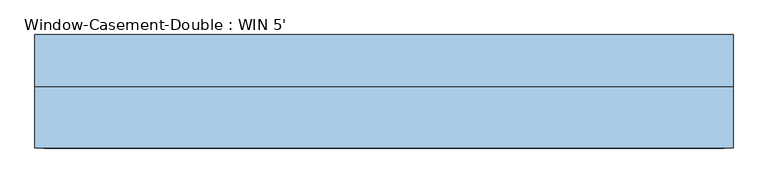
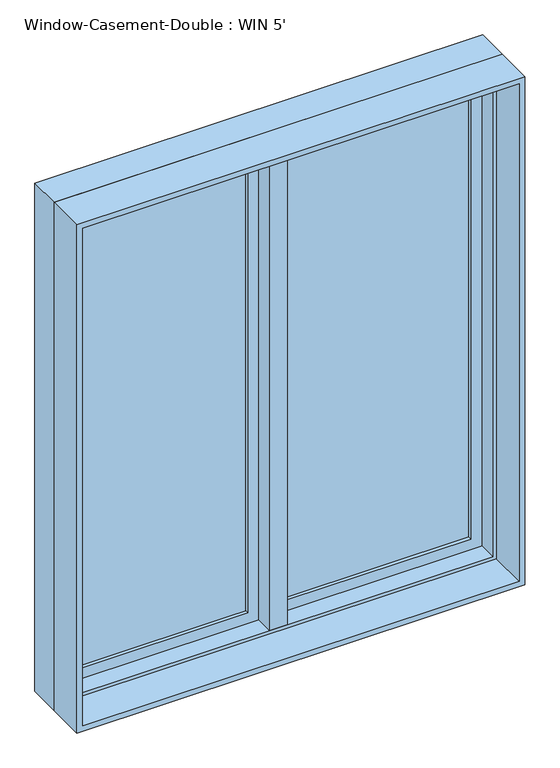
"""IFC4 building model written with IfcOpenShell, lengths in millimetres: window geometry, Window-Casement-Double : WIN 5'."""

from ifc_helpers import new_model, si_unit, frame, origin, place, context, project, spatial, polyline, outline, extrude, faceted_brep, source, transform, mapped, element, save


def window_casement_double_win_5_f93960c7(model_context):
    return source(origin(), model_context, "Body", "SolidModel", [
        faceted_brep([(9.525, 133.35, 2730.5), (-9.525, 133.35, 2730.5), (-9.525, 82.55, 2730.5), (9.525, 82.55, 2730.5), (9.525, 133.35, 927.1), (9.525, 82.55, 927.1), (-9.525, 82.55, 927.1), (-9.525, 133.35, 927.1), (-9.525, 82.55, 946.15), (-9.525, 82.55, 2711.45), (-30.1625, 82.55, 946.15), (-30.1625, 82.55, 2711.45), (-30.1625, 19.05, 946.15), (-30.1625, 19.05, 2711.45), (30.1625, 19.05, 946.15), (30.1625, 19.05, 2711.45), (30.1625, 82.55, 946.15), (30.1625, 82.55, 2711.45), (9.525, 82.55, 946.15), (9.525, 82.55, 2711.45)], [[[0, 1, 2, 3]], [[4, 5, 6, 7]], [[1, 0, 4, 7]], [[2, 1, 7, 6, 8, 9]], [[9, 8, 10, 11]], [[11, 10, 12, 13]], [[13, 12, 14, 15]], [[15, 14, 16, 17]], [[17, 16, 18, 19]], [[0, 3, 19, 18, 5, 4]], [[18, 8, 6, 5]], [[9, 19, 3, 2]], [[8, 18, 16, 14, 12, 10]], [[19, 9, 11, 13, 15, 17]]]),
        extrude(outline(polyline([(-66.675, 114.3), (-66.675, 107.95), (-692.15, 107.95), (-692.15, 114.3), (-66.675, 114.3)])), frame((0.0, 0.0, 984.25), z_axis=(0.0, 0.0, 1.0), x_axis=(1.0, 0.0, 0.0)), (0.0, 0.0, 1.0), 1689.1),
        extrude(outline(polyline([(-692.15, 95.25), (-692.15, 101.6), (-66.675, 101.6), (-66.675, 95.25), (-692.15, 95.25)])), frame((0.0, 0.0, 984.25), z_axis=(0.0, 0.0, 1.0), x_axis=(1.0, 0.0, 0.0)), (0.0, 0.0, 1.0), 1689.1),
        extrude(outline(polyline([(692.15, 114.3), (692.15, 107.95), (66.675, 107.95), (66.675, 114.3), (692.15, 114.3)])), frame((0.0, 0.0, 984.25), z_axis=(0.0, 0.0, 1.0), x_axis=(1.0, 0.0, 0.0)), (0.0, 0.0, 1.0), 1689.1),
        extrude(outline(polyline([(66.675, 95.25), (66.675, 101.6), (692.15, 101.6), (692.15, 95.25), (66.675, 95.25)])), frame((0.0, 0.0, 984.25), z_axis=(0.0, 0.0, 1.0), x_axis=(1.0, 0.0, 0.0)), (0.0, 0.0, 1.0), 1689.1),
        extrude(outline(polyline([(2730.5, -749.3), (927.1, -749.3), (927.1, -9.525), (2730.5, -9.525), (2730.5, -749.3)]), holes=[polyline([(2673.35, -66.675), (984.25, -66.675), (984.25, -692.15), (2673.35, -692.15), (2673.35, -66.675)])]), frame((0.0, 82.55, 0.0), z_axis=(0.0, 1.0, 0.0), x_axis=(0.0, 0.0, 1.0)), (0.0, 0.0, 1.0), 44.45),
        extrude(outline(polyline([(927.1, 749.3), (2730.5, 749.3), (2730.5, 9.525), (927.1, 9.525), (927.1, 749.3)]), holes=[polyline([(984.25, 66.675), (2673.35, 66.675), (2673.35, 692.15), (984.25, 692.15), (984.25, 66.675)])]), frame((0.0, 82.55, 0.0), z_axis=(0.0, 1.0, 0.0), x_axis=(0.0, 0.0, 1.0)), (0.0, 0.0, 1.0), 44.45),
        extrude(outline(polyline([(2743.2, -762.0), (914.4, -762.0), (914.4, 762.0), (2743.2, 762.0), (2743.2, -762.0)]), holes=[polyline([(2724.15, 742.95), (933.45, 742.95), (933.45, -742.95), (2724.15, -742.95), (2724.15, 742.95)])]), frame((0.0, -114.3, 0.0), z_axis=(0.0, 1.0, 0.0), x_axis=(0.0, 0.0, 1.0)), (0.0, 0.0, 1.0), 133.35),
        faceted_brep([(730.25, 82.55, 2711.45), (730.25, 19.05, 2711.45), (-730.25, 19.05, 2711.45), (-730.25, 82.55, 2711.45), (749.3, 133.35, 2730.5), (749.3, 82.55, 2730.5), (-749.3, 82.55, 2730.5), (-749.3, 133.35, 2730.5), (762.0, 19.05, 2743.2), (762.0, 133.35, 2743.2), (-762.0, 133.35, 2743.2), (-762.0, 19.05, 2743.2), (-730.25, 19.05, 946.15), (-730.25, 82.55, 946.15), (-749.3, 82.55, 927.1), (-749.3, 133.35, 927.1), (-762.0, 133.35, 914.4), (-762.0, 19.05, 914.4), (730.25, 19.05, 946.15), (730.25, 82.55, 946.15), (749.3, 82.55, 927.1), (749.3, 133.35, 927.1), (762.0, 133.35, 914.4), (762.0, 19.05, 914.4)], [[[0, 1, 2, 3]], [[4, 5, 6, 7]], [[8, 9, 10, 11]], [[3, 2, 12, 13]], [[7, 6, 14, 15]], [[11, 10, 16, 17]], [[13, 12, 18, 19]], [[15, 14, 20, 21]], [[17, 16, 22, 23]], [[11, 17, 23, 8], [1, 18, 12, 2]], [[19, 18, 1, 0]], [[5, 20, 14, 6], [3, 13, 19, 0]], [[21, 20, 5, 4]], [[23, 22, 9, 8]], [[9, 22, 16, 10], [7, 15, 21, 4]]]),
    ])


if __name__ == "__main__":
    model = new_model("IFC4")
    model_context = context("Model", 3, world=origin())
    ifc_project = project(units=[si_unit("LENGTHUNIT", "METRE", prefix="MILLI")], contexts=[model_context])
    site = spatial("IfcSite", under=ifc_project)
    building = spatial("IfcBuilding", under=site)
    placement = place(None, origin())
    window_casement_double_win_5_shape = window_casement_double_win_5_f93960c7(model_context)
    element("IfcWindow", 1, ObjectType="Window-Casement-Double : WIN 5'", at=placement, inside=building, context=model_context, shape_type="MappedRepresentation", body=[
        mapped(window_casement_double_win_5_shape, transform((0.0, 0.0, 0.0), x_axis=(1.0, 0.0, 0.0), y_axis=(0.0, 1.0, 0.0), z_axis=(0.0, 0.0, 1.0))),
    ])
    save(model, "model.ifc")

# Revit data of these elements
# Type "Window-Casement-Double : WIN 5'"
#   Type Mark = "18"
#   Fire Rating = "0.5h"
#   Assembly Code = "B2020100"
#   Analytic Construction = "Double glazing - domestic"
#   Frame Extension [instance default] = 0' - 0 1/4"
#   Window Inset [instance default] = 0' - 0"
#   Wall Thickness [instance default] = 0' - 6"
#   Interior Wall Closure [instance default] = 0' - 2 1/4"
#   Half Width = 2' - 6"
#   Visual Light Transmittance = 0.81
#   Thermal Resistance (R) = 1.8146 (h·ft²·°F)/BTU
#   Solar Heat Gain Coefficient = 0.76
#   Rough Width = 5' - 0 1/2"
#   Rough Height = 6' - 0 1/2"
#   Height = 6' - 0"
#   Heat Transfer Coefficient (U) = 0.5511 BTU/(h·ft²·°F)
#   Exterior Wall Closure [instance default] = 0' - 1 1/4"
#   Extension Jamb [instance default] = 0' - 2 1/4"
#   Default Sill Height = 3' - 0"
#   Width = 5' - 0"
#   Muntin Visibility = yes
#   Interior Trim Visibility [instance default] = yes
#   Exterior Trim Visibility [instance default] = yes
#   Extension Jamb Visibility [instance default] = yes
#   Interior Trim Material = Wood - Stained
#   Muntin Pattern = Muntin Pattern_2x2 : Muntin Pattern_2x2
#   Interior Trim = Trim-Window-Interior-Flat : Picture Frame
#   Interior Frame Material = Wood - Stained
#   Glass Panel Material = Glass
#   Exterior Trim Material = Clad - White
#   Exterior Trim = Trim-Window-Exterior-Flat : with Sill
#   Exterior Frame Material = Clad - White
#   Wall Closure = (empty or 0)
# Element 1 (IfcWindow, "Window-Casement-Double : WIN 5'")
#   Wall Thickness = 0' - 9"
#   Extension Jamb = 0' - 5 1/4"
#   Materials on its faces: "Wood - Stained", "Glass", "Clad - White"
# Materials
#   "Wood - Stained": class "Wood", colour RGB 224 178 126, transparency 0, Cost = 0
#   "Glass": class "Glass", colour RGB 0 128 192, transparency 0.75, Description = "Soda Lime Glass", Cost = 0
#   "Clad - White": class "Wood", colour RGB 242 242 238, transparency 0, Cost = 0
